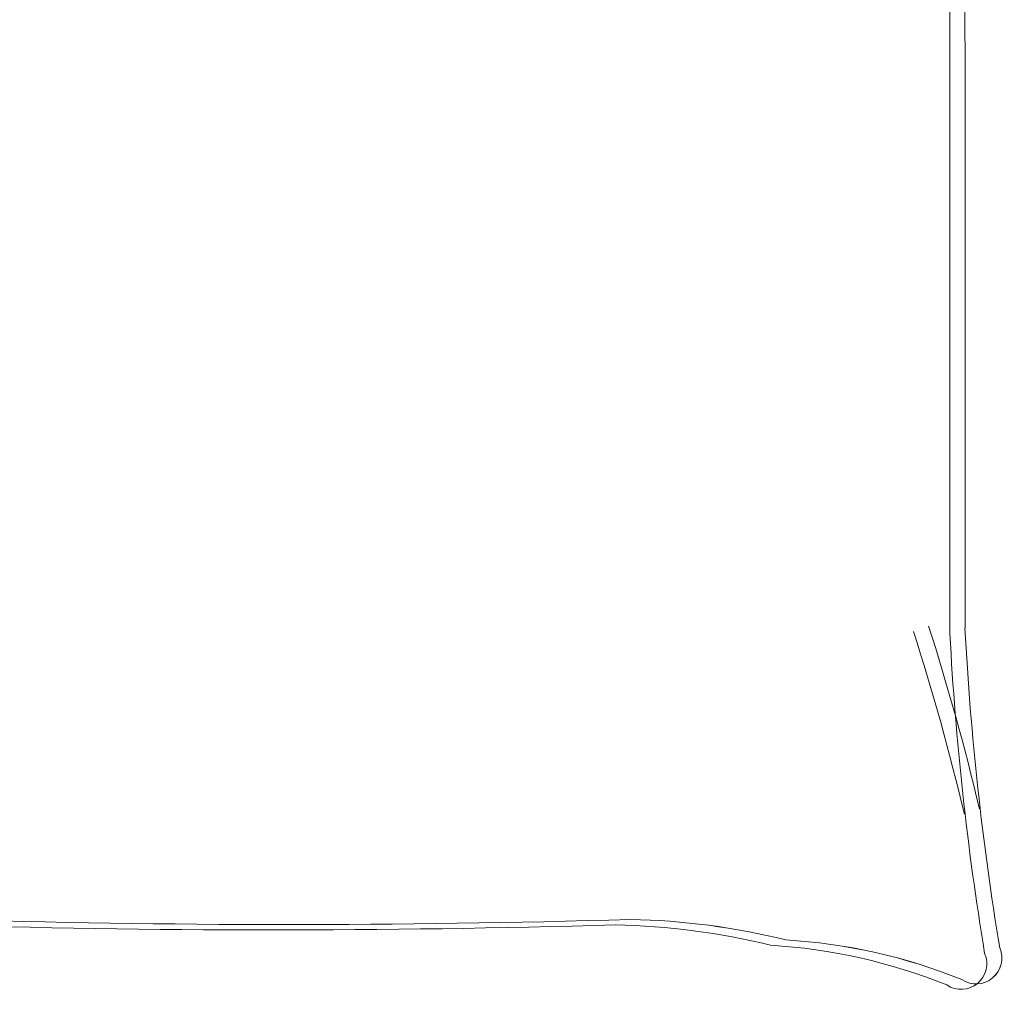
# Model space of a CAD drawing. Units: inches. Extents: x 1885 to 2748, y 783 to 2421.
# Tile 11 of 117: x 2017 to 2059, y 1137 to 1178. Entities that reach past the tile are written whole.
import ezdxf

# ---------------------------------------------------------------- set-up
doc = ezdxf.new("R2010")
doc.units = ezdxf.units.IN
doc.layers.add('A-FURN', color=8, linetype='Continuous', lineweight=13)

# ---------------------------------------------------------------- blocks, each defined once
blk = doc.blocks.new('BED-DOUBLE')
for p, q in [((28.389, 53.095), (25.139, 49.389)), ((28.389, 53.094), (25.139, 49.389)), ((30.133, 53.174), (28.389, 53.095, 3.871)), ((30.133, 53.174), (28.389, 53.094, 3.871)), ((29.008, 51.558), (28.389, 53.095)), ((29.008, 51.557), (28.389, 53.094)), ((27.749, 52.866), (24.499, 49.161)), ((27.75, 52.866), (24.499, 49.161)), ((29.494, 52.946), (27.749, 52.866, 3.871)), ((28.369, 51.329), (27.749, 52.866)), ((29.494, 52.945), (27.75, 52.866, 3.871)), ((28.369, 51.329), (27.75, 52.866)), ((0.004, 51.493), (0.643, 51.492)), ((0.004, 3.474), (0.004, 51.493)), ((0.643, 51.493), (27.253, 51.493)), ((0.643, 51.492), (27.253, 51.492)), ((2.177, 3.702), (2.177, 51.493)), ((2.177, 3.702), (2.177, 51.492)), ((28.059, 48.232), (28.369, 51.329)), ((28.059, 48.231), (28.369, 51.329)), ((28.698, 48.46), (29.008, 51.558)), ((28.698, 48.46), (29.008, 51.557)), ((0.004, 51.264), (26.614, 51.264)), ((0.004, 51.264), (26.614, 51.264)), ((1.537, 3.474), (1.537, 51.264)), ((1.537, 3.474), (1.537, 51.264)), ((17.216, 50.925), (14.077, 50.15)), ((17.216, 50.925), (14.077, 50.15)), ((16.812, 45.794), (17.216, 50.925)), ((16.812, 45.793), (17.216, 50.925)), ((6.411, 49.96), (8.981, 50.556)), ((6.411, 49.96), (8.981, 50.555)), ((8.981, 50.556), (10.027, 50.042)), ((8.981, 50.555), (10.027, 50.041)), ((16.576, 50.697), (13.438, 49.922)), ((16.576, 50.697), (13.438, 49.921)), ((16.173, 45.565), (16.576, 50.697)), ((16.173, 45.565), (16.576, 50.697)), ((2.561, 50.111), (2.464, 44.708)), ((2.561, 50.11), (2.464, 44.708)), ((2.561, 50.111), (5.771, 49.732)), ((2.561, 50.11), (5.771, 49.732)), ((3.2, 50.339), (3.103, 44.937)), ((3.2, 50.339), (3.103, 44.936)), ((3.2, 50.339), (6.411, 49.96)), ((3.2, 50.339), (6.411, 49.96)), ((5.771, 49.732), (8.342, 50.327)), ((5.771, 49.732), (8.342, 50.327)), ((11.832, 50.111), (8.261, 49.308)), ((11.832, 50.111), (8.261, 49.308)), ((8.342, 50.327), (9.388, 49.813)), ((8.342, 50.327), (9.388, 49.813)), ((12.472, 50.339), (8.9, 49.537)), ((12.472, 50.339), (8.9, 49.536)), ((13.438, 49.922), (11.832, 50.111)), ((13.438, 49.921), (11.832, 50.111)), ((14.077, 50.15), (12.472, 50.339)), ((14.077, 50.15), (12.472, 50.339)), ((8.261, 49.308), (5.582, 48.127)), ((8.261, 49.308), (5.582, 48.127)), ((8.9, 49.537), (6.221, 48.355)), ((8.9, 49.536), (6.221, 48.355)), ((25.139, 49.389), (22.972, 46.447)), ((25.139, 49.389), (22.972, 46.447)), ((24.499, 49.161), (22.332, 46.218)), ((24.499, 49.161), (22.332, 46.218)), ((29.008, 44.588), (28.698, 48.46)), ((29.008, 44.588), (28.698, 48.46)), ((28.369, 44.36), (28.059, 48.232)), ((28.369, 44.36), (28.059, 48.231)), ((22.972, 46.447), (20.96, 40.871)), ((22.972, 46.447), (20.96, 40.871)), ((3.103, 44.937), (3.185, 45.939)), ((3.103, 44.936), (3.185, 45.939)), ((3.185, 45.939), (3.712, 42.141)), ((3.185, 45.939), (3.712, 42.141)), ((22.332, 46.218), (20.32, 40.643)), ((22.332, 46.218), (20.32, 40.643)), ((2.464, 44.708), (2.546, 45.711)), ((2.464, 44.708), (2.546, 45.711)), ((2.546, 45.711), (3.073, 41.913)), ((2.546, 45.711), (3.073, 41.913)), ((16.73, 43.605), (16.173, 45.565)), ((16.73, 43.605), (16.173, 45.565)), ((17.369, 43.833), (16.812, 45.794)), ((17.369, 43.833), (16.812, 45.793)), ((28.833, 40.953), (28.369, 44.36)), ((28.833, 40.952), (28.369, 44.36)), ((29.472, 41.181), (29.008, 44.588)), ((29.472, 41.181), (29.008, 44.588)), ((16.938, 36.823), (17.369, 43.833)), ((16.938, 36.823), (17.369, 43.833)), ((16.299, 36.595), (16.73, 43.605)), ((16.299, 36.595), (16.73, 43.605)), ((3.712, 42.141), (5.065, 36.722)), ((3.712, 42.141), (5.065, 36.722)), ((3.073, 41.913), (4.426, 36.494)), ((3.073, 41.913), (4.426, 36.493)), ((20.96, 40.871), (18.026, 32.533)), ((20.96, 40.871), (18.026, 32.533)), ((29.762, 38.939), (28.833, 40.953)), ((29.762, 38.939), (28.833, 40.952)), ((30.401, 39.168), (29.472, 41.181)), ((30.401, 39.167), (29.472, 41.181)), ((20.32, 40.643), (17.387, 32.305)), ((20.32, 40.643), (17.387, 32.305)), ((79.249, 15.062), (79.249, 39.676)), ((79.249, 15.062), (79.249, 39.676)), ((79.888, 15.29), (79.888, 39.904)), ((79.888, 15.29), (79.888, 39.904)), ((4.317, 39.427), (3.721, 37.362)), ((4.317, 39.427), (3.721, 37.362)), ((3.677, 39.199), (3.082, 37.134)), ((3.677, 39.199), (3.082, 37.134)), ((30.381, 36.461), (29.762, 38.939)), ((30.381, 36.461), (29.762, 38.939)), ((31.02, 36.69), (30.401, 39.168)), ((31.02, 36.689), (30.401, 39.167)), ((3.082, 37.134), (2.541, 34.203)), ((3.082, 37.134), (2.541, 34.203)), ((3.721, 37.362), (3.18, 34.432)), ((3.721, 37.362), (3.18, 34.431)), ((16.271, 32.791), (16.938, 36.823)), ((16.272, 32.791), (16.938, 36.823)), ((15.632, 32.563), (16.299, 36.595)), ((15.632, 32.563), (16.299, 36.595)), ((24.519, 34.676), (29.008, 36.38)), ((24.519, 34.676), (29.008, 36.38)), ((28.369, 36.152), (30.381, 36.461)), ((28.369, 36.151), (30.381, 36.461)), ((29.008, 36.38), (31.02, 36.69)), ((29.008, 36.38), (31.02, 36.689)), ((23.88, 34.448), (28.369, 36.152)), ((23.88, 34.448), (28.369, 36.151)), ((18.026, 30.486), (24.519, 34.676)), ((18.026, 30.486), (24.519, 34.676)), ((2.541, 34.203), (2.561, 33.882)), ((2.541, 34.203), (2.561, 33.882)), ((3.18, 34.432), (3.2, 34.111)), ((3.18, 34.431), (3.2, 34.11)), ((17.387, 30.258), (23.88, 34.448)), ((17.387, 30.258), (23.88, 34.448)), ((2.561, 33.882), (2.982, 29.454)), ((2.561, 33.882), (2.982, 29.454)), ((3.2, 34.111), (3.622, 29.683)), ((3.2, 34.11), (3.622, 29.683)), ((16.743, 30.749), (15.458, 33.819)), ((16.743, 30.749), (15.458, 33.819)), ((17.382, 30.977), (16.097, 34.048)), ((17.382, 30.977), (16.097, 34.048)), ((17.536, 28.525), (17.382, 30.977)), ((17.536, 28.524), (17.382, 30.977)), ((16.896, 28.296), (16.743, 30.749)), ((16.896, 28.296), (16.743, 30.749)), ((3.622, 29.683), (3.135, 28.204)), ((3.622, 29.683), (3.135, 28.204)), ((2.982, 29.454), (2.495, 27.976)), ((2.982, 29.454), (2.495, 27.975)), ((14.86, 28.357), (17.536, 28.525)), ((14.86, 28.357), (17.536, 28.524)), ((2.495, 27.976), (7.871, 27.732)), ((2.495, 27.975), (7.871, 27.732)), ((3.135, 28.204), (8.51, 27.961)), ((3.135, 28.204), (8.51, 27.96)), ((8.51, 27.961), (11.721, 27.582)), ((8.51, 27.96), (11.721, 27.582)), ((12.38, 27.435), (14.22, 28.129)), ((12.38, 27.434), (14.22, 28.129)), ((13.02, 27.663), (14.86, 28.357)), ((13.02, 27.663), (14.86, 28.357)), ((14.22, 28.129), (16.896, 28.296)), ((14.22, 28.129), (16.896, 28.296)), ((7.871, 27.732), (11.082, 27.354)), ((7.871, 27.732), (11.082, 27.353)), ((11.721, 27.582), (13.02, 27.663)), ((11.721, 27.582), (13.02, 27.663)), ((7.224, 26.56), (10.404, 27.138)), ((7.224, 26.559), (10.405, 27.137)), ((7.863, 26.788), (11.044, 27.366)), ((7.863, 26.788), (11.044, 27.366)), ((10.404, 27.138), (11.706, 27.138)), ((10.405, 27.137), (11.706, 27.137)), ((11.044, 27.366), (12.345, 27.366)), ((11.044, 27.366), (12.345, 27.366)), ((11.082, 27.354), (12.38, 27.435)), ((11.082, 27.353), (12.38, 27.434)), ((11.706, 27.138), (13.585, 26.56)), ((11.706, 27.137), (13.585, 26.559)), ((12.345, 27.366), (14.225, 26.788)), ((12.345, 27.366), (14.225, 26.788)), ((2.513, 26.21), (7.863, 26.788)), ((2.513, 26.209), (7.863, 26.788)), ((14.225, 26.788), (16.906, 26.788)), ((14.225, 26.788), (16.906, 26.788)), ((16.906, 26.788), (16.906, 24.33)), ((16.906, 26.788), (16.906, 24.33)), ((1.874, 25.981), (7.224, 26.56)), ((1.874, 25.981), (7.224, 26.559)), ((13.585, 26.56), (16.267, 26.56)), ((13.585, 26.559), (16.267, 26.559)), ((16.267, 26.56), (16.267, 24.102)), ((16.267, 26.559), (16.267, 24.102)), ((2.452, 24.536), (1.874, 25.981)), ((2.452, 24.535), (1.874, 25.981)), ((3.091, 24.764), (2.513, 26.21)), ((3.091, 24.764), (2.513, 26.209)), ((2.947, 20.319), (3.091, 24.764)), ((2.947, 20.318), (3.091, 24.764)), ((16.812, 19.611), (17.216, 24.743)), ((16.812, 19.611), (17.216, 24.743)), ((2.308, 20.09), (2.452, 24.536)), ((2.308, 20.09), (2.452, 24.535)), ((16.906, 24.33), (15.815, 21.186)), ((16.906, 24.33), (15.815, 21.186)), ((16.173, 19.383), (16.576, 24.515)), ((16.173, 19.382), (16.576, 24.514)), ((16.267, 24.102), (15.176, 20.957)), ((16.267, 24.102), (15.176, 20.957)), ((2.308, 19.769), (2.308, 20.09)), ((2.308, 19.768), (2.308, 20.09)), ((2.947, 19.997), (2.947, 20.319)), ((2.947, 19.997), (2.947, 20.318)), ((3.031, 16.877), (2.308, 19.769)), ((3.031, 16.877), (2.308, 19.768)), ((3.67, 17.106), (2.947, 19.997)), ((3.67, 17.105), (2.947, 19.997)), ((17.369, 17.651), (16.812, 19.611)), ((17.369, 17.65), (16.812, 19.611)), ((16.73, 17.422), (16.173, 19.383)), ((16.73, 17.422), (16.173, 19.382)), ((3.32, 12.107), (4.332, 17.6)), ((3.32, 12.107), (4.332, 17.6)), ((3.959, 12.335), (4.971, 17.829)), ((3.959, 12.335), (4.971, 17.828)), ((16.938, 10.641), (17.369, 17.651)), ((16.938, 10.64), (17.369, 17.65)), ((4.393, 15.082), (3.67, 17.106)), ((4.393, 15.082), (3.67, 17.105)), ((16.299, 10.412), (16.73, 17.422)), ((16.299, 10.412), (16.73, 17.422)), ((3.753, 14.854), (3.031, 16.877)), ((3.753, 14.853), (3.031, 16.877)), ((3.031, 8.284), (3.32, 12.107)), ((3.031, 8.283), (3.32, 12.107)), ((3.67, 8.512), (3.959, 12.335)), ((3.67, 8.512), (3.959, 12.335)), ((16.271, 6.609), (16.938, 10.641)), ((16.272, 6.609), (16.938, 10.64)), ((16.938, 10.641), (17.261, 9.508)), ((16.938, 10.64), (17.261, 9.507)), ((15.632, 6.38), (16.299, 10.412)), ((15.632, 6.38), (16.299, 10.412)), ((16.299, 10.412), (16.622, 9.279)), ((16.299, 10.412), (16.622, 9.279)), ((16.622, 9.279), (17.345, 4.183)), ((16.622, 9.279), (17.345, 4.182)), ((17.261, 9.508), (17.984, 4.411)), ((17.261, 9.507), (17.984, 4.411)), ((3.652, 8.407), (3.67, 8.512)), ((3.652, 8.406), (3.67, 8.512)), ((3.981, 4.126), (3.652, 8.407)), ((3.981, 4.125), (3.652, 8.406)), ((3.012, 8.178), (3.031, 8.284)), ((3.012, 8.178), (3.031, 8.283)), ((3.342, 3.897), (3.012, 8.178)), ((3.342, 3.897), (3.012, 8.178)), ((9.598, 5.278), (6.851, 6.29)), ((9.598, 5.278), (6.851, 6.29)), ((8.959, 5.05), (6.211, 6.062)), ((8.959, 5.05), (6.211, 6.061)), ((12.573, 4.472), (8.959, 5.05)), ((12.573, 4.471), (8.959, 5.05)), ((13.213, 4.7), (9.598, 5.278)), ((13.213, 4.7), (9.598, 5.278)), ((3.959, 4.122), (7.14, 4.7)), ((3.959, 4.121), (7.14, 4.7)), ((7.14, 4.7), (9.743, 4.266)), ((7.14, 4.7), (9.743, 4.266)), ((9.103, 4.038), (10.115, 4.616)), ((9.103, 4.038), (10.115, 4.616)), ((9.743, 4.266), (10.755, 4.845)), ((9.743, 4.266), (10.755, 4.844)), ((14.164, 4.761), (12.573, 4.472)), ((14.164, 4.76), (12.573, 4.471)), ((14.803, 4.989), (13.213, 4.7)), ((14.803, 4.989), (13.213, 4.7)), ((17.345, 4.183), (14.164, 4.761)), ((17.345, 4.182), (14.164, 4.76)), ((17.984, 4.411), (14.803, 4.989)), ((17.984, 4.411), (14.803, 4.989)), ((3.32, 3.893), (6.501, 4.472)), ((3.32, 3.893), (6.501, 4.471)), ((6.501, 4.472), (9.103, 4.038)), ((6.501, 4.471), (9.103, 4.038)), ((18.114, 3.474), (0.004, 3.474)), ((18.114, 3.474), (0.004, 3.474)), ((18.753, 3.702), (0.643, 3.702)), ((18.753, 3.702), (0.643, 3.702))]:
    blk.add_line(p, q)
for centre, radius, start, end in [((68.67, 76.156), 23.065, 267.4714, 296.4681), ((68.67, 76.156), 23.065, 267.4714, 296.4681), ((69.309, 76.384), 23.065, 267.4714, 296.4681), ((69.309, 76.384), 23.065, 267.4714, 296.4681), ((78.874, 54.409), 1.102, 332.6588, 86.02), ((78.874, 54.408), 1.102, 332.6588, 86.02), ((79.513, 54.637), 1.102, 332.6588, 86.02), ((79.513, 54.637), 1.102, 332.6588, 86.02), ((212.28, 41.151), 133.04, 174.4998, 180.63509), ((212.28, 41.15), 133.04, 174.4998, 180.63509), ((212.92, 41.379), 133.04, 174.4998, 180.63509), ((212.92, 41.379), 133.04, 174.4998, 180.63509), ((36.319, 182.265), 129.499, 266.97912, 273.83645), ((36.319, 182.264), 129.499, 266.97912, 273.83645), ((-6.013, 51.554), 36.183, 349.8763, 2.5657), ((-6.013, 51.554), 36.183, 349.8763, 2.5657), ((36.958, 182.493), 129.499, 266.97912, 273.83645), ((36.958, 182.493), 129.499, 266.97912, 273.83645), ((67.825, -4508.745), 4561.858, 90.002168, 90.286887), ((67.825, -4508.745), 4561.858, 90.002168, 90.286887), ((68.464, -4508.516), 4561.858, 90.002168, 90.286887), ((68.464, -4508.517), 4561.858, 90.002168, 90.286887), ((-6.653, 51.326), 36.183, 349.8763, 2.5657), ((-6.653, 51.326), 36.183, 349.8763, 2.5657), ((35.709, 43.971), 6.224, 168.6608, 203.7384), ((35.709, 43.97), 6.224, 168.6608, 203.7384), ((35.07, 43.742), 6.224, 168.6608, 203.7384), ((35.07, 43.742), 6.224, 168.6608, 203.7384), ((2.125, 31.381), 29.654, 10.6617, 19.8806), ((2.125, 31.381), 29.654, 10.6617, 19.8806), ((1.486, 31.152), 29.654, 10.6617, 19.8806), ((1.486, 31.152), 29.654, 10.6617, 19.8806), ((31.082, 36.863), 0.185, 250.2464, 1.1377), ((31.082, 36.863), 0.185, 250.2464, 1.1377), ((156.959, 17.983), 129.02, 171.78449, 186.90062), ((156.959, 17.983), 129.02, 171.78449, 186.90062), ((30.443, 36.635), 0.185, 250.2464, 1.1377), ((30.443, 36.635), 0.185, 250.2464, 1.1377), ((156.32, 17.754), 129.02, 171.78449, 186.90062), ((156.32, 17.754), 129.02, 171.78449, 186.90062), ((182.056, 21.358), 164.969, 176.08655, 186.78213), ((182.056, 21.357), 164.969, 176.08655, 186.78213), ((182.695, 21.586), 164.969, 176.08655, 186.78213), ((182.695, 21.586), 164.969, 176.08655, 186.78213), ((-23.708, -17.223), 106.459, 13.38322, 17.70533), ((-23.708, -17.223), 106.459, 13.38322, 17.70533), ((-23.069, -16.995), 106.459, 13.38322, 17.70533), ((-23.069, -16.995), 106.459, 13.38322, 17.70533), ((200.841, 21.425), 121.759, 182.99578, 189.40907), ((200.841, 21.425), 121.759, 182.99578, 189.40907), ((201.48, 21.654), 121.759, 182.99578, 189.40907), ((201.48, 21.654), 121.759, 182.99578, 189.40907), ((31.817, -167.08), 170.11, 88.4762, 91.00819), ((31.817, -167.081), 170.11, 88.4762, 91.00819), ((51.257, 485.049), 482.31, 268.22771, 271.71854), ((51.257, 485.049), 482.31, 268.22771, 271.71854), ((65.158, -26.672), 29.634, 76.0648, 88.9113), ((65.158, -26.673), 29.634, 76.0648, 88.9113), ((31.177, -167.309), 170.11, 88.4762, 91.00819), ((31.177, -167.309), 170.11, 88.4762, 91.00819), ((50.617, 484.821), 482.31, 268.22771, 271.71854), ((50.617, 484.821), 482.31, 268.22771, 271.71854), ((64.519, -26.901), 29.634, 76.0648, 88.9113), ((64.519, -26.901), 29.634, 76.0648, 88.9113), ((20.1, 85.16), 83.306, 268.72178, 275.60397), ((20.1, 85.16), 83.306, 268.72178, 275.60397), ((20.739, 85.389), 83.306, 268.72178, 275.60397), ((20.739, 85.389), 83.306, 268.72178, 275.60397), ((70.919, -21.432), 23.562, 67.9751, 86.652), ((70.919, -21.433), 23.562, 67.9751, 86.652), ((70.279, -21.661), 23.562, 67.9751, 86.652), ((70.279, -21.661), 23.562, 67.9751, 86.652), ((80.361, 1.315), 1.089, 236.1736, 23.4781), ((80.361, 1.314), 1.089, 236.1736, 23.4781), ((79.721, 1.086), 1.089, 236.1736, 23.4781), ((79.721, 1.086), 1.089, 236.1736, 23.4781)]:
    blk.add_arc(centre, radius, start, end)

msp = doc.modelspace()

# ---------------------------------------------------------------- block references
at = {"layer": 'A-FURN'}
msp.add_blockref('BED-DOUBLE', (1977.555, 1137.199), dxfattribs=at)

doc.saveas('drawing.dxf')
